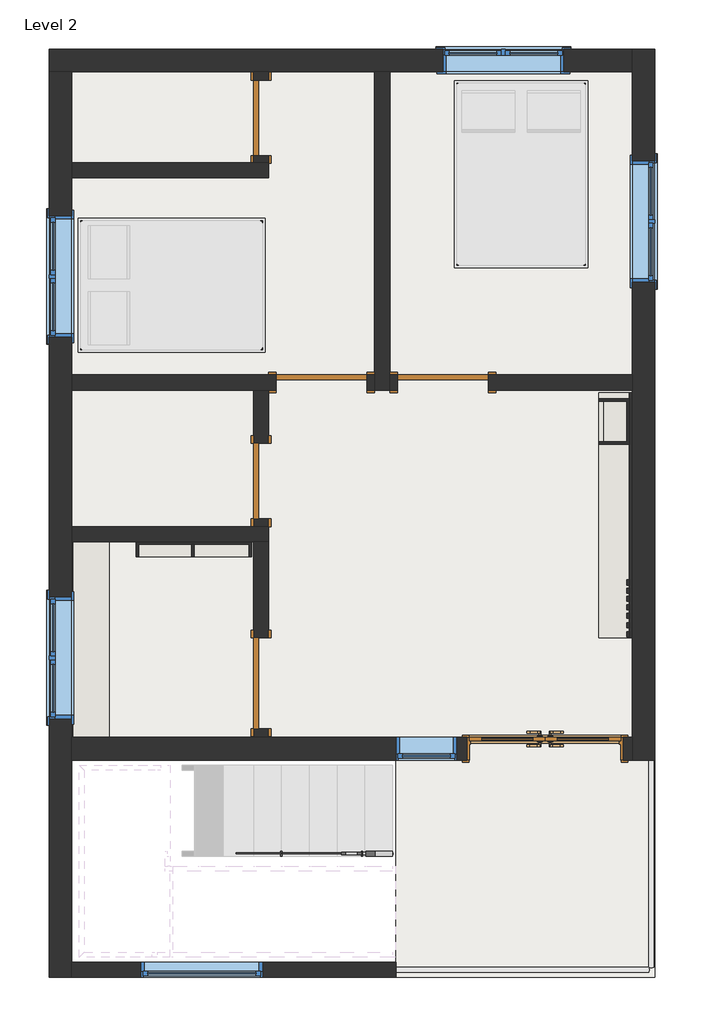
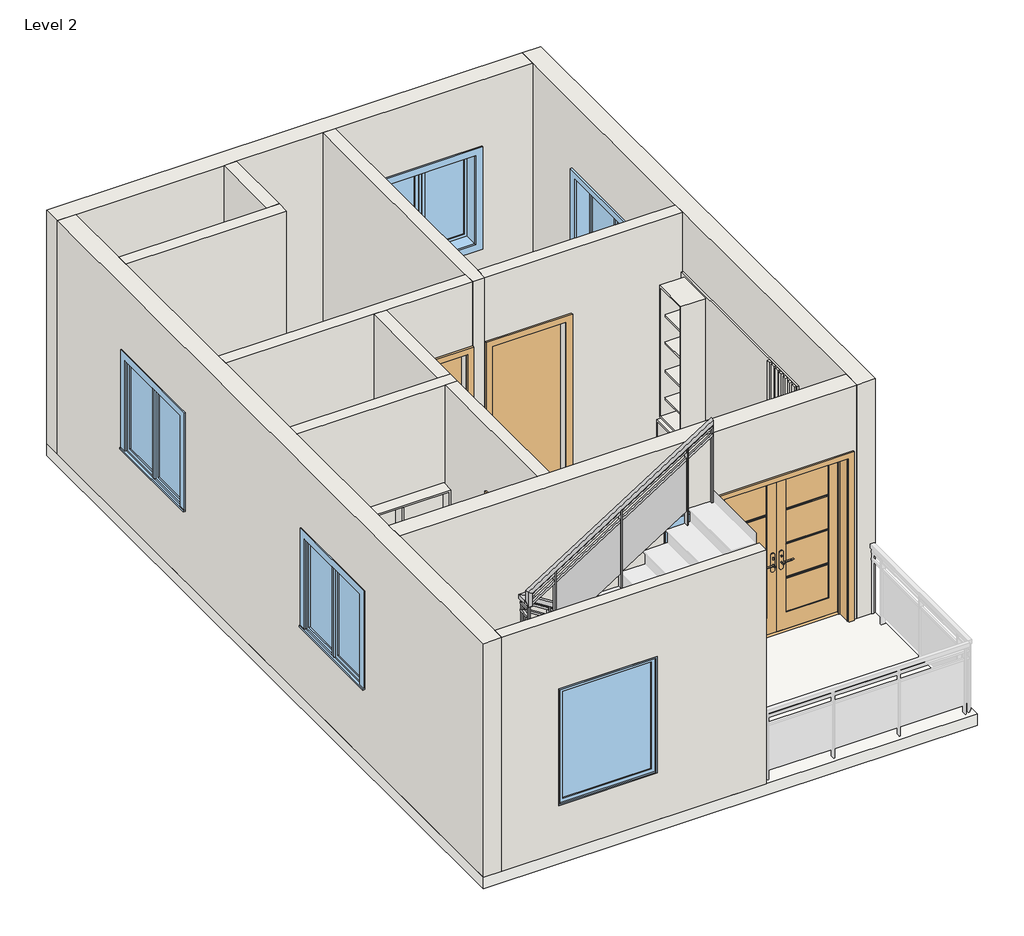
# One storey, part 1 of 2: 15 walls, 6 doors, 6 windows, 1 railing, 1 slab.
"""IFC4 building model written with IfcOpenShell, lengths in millimetres."""

from ifc_helpers import new_model, si_unit, frame, origin, place, context, project, spatial, polyline, outline, extrude, faceted_brep, transform, mapped, element, save
from components import m_door_exterior_double_full_glass_wood_clad_1524_x_2134mm_606f56d5, single_flush_2_5_e2b13fe9, door_686f89d2, door_16372e1c, walls_3_walls_1_7bd47e67, walls_4_walls_2_ccd45d7e, window_534dcd48, window_fc882ab3, fixed_4_86eadd64

model = new_model("IFC4")

# Units and contexts
model_context = context("Model", 3, world=origin())
ifc_project = project(units=[si_unit("LENGTHUNIT", "METRE", prefix="MILLI")], contexts=[model_context])

# Site, building, storey
site = spatial("IfcSite", under=ifc_project)
building = spatial("IfcBuilding", under=site)
storey = spatial("IfcBuildingStorey", under=building, Name="Level 2", Elevation=3200.4)

# Doors
placement = place(None, origin())
m_door_exterior_double_full_glass_wood_clad_1524_x_2134mm_shape = m_door_exterior_double_full_glass_wood_clad_1524_x_2134mm_606f56d5(model_context)
element("IfcDoor", 1, ObjectType="M_Door-Exterior-Double-Full Glass-Wood_Clad : 1524 x 2134mm", at=placement, inside=storey, context=model_context, shape_type="MappedRepresentation", body=[
    mapped(m_door_exterior_double_full_glass_wood_clad_1524_x_2134mm_shape, transform((-1706.0473712, -4701.782676, 3200.4), x_axis=(1.0, 0.0, 0.0), y_axis=(0.0, 1.0, 0.0), z_axis=(0.0, 0.0, 1.0))),
])
single_flush_2_5_shape = single_flush_2_5_e2b13fe9(model_context)
element("IfcDoor", 2, ObjectType="Single-Flush : 2.5'", at=placement, inside=storey, context=model_context, shape_type="MappedRepresentation", body=[
    mapped(single_flush_2_5_shape, transform((-4563.5473712, -2012.557676, 3200.4), x_axis=(0.0, -1.0, 0.0), y_axis=(1.0, 0.0, 0.0), z_axis=(0.0, 0.0, 1.0))),
])
element("IfcDoor", 3, ObjectType="Single-Flush : 2.5'", at=placement, inside=storey, context=model_context, shape_type="MappedRepresentation", body=[
    mapped(single_flush_2_5_shape, transform((-4563.5473712, 1638.692324, 3200.4), x_axis=(0.0, -1.0, 0.0), y_axis=(1.0, 0.0, 0.0), z_axis=(0.0, 0.0, 1.0))),
])
door_shape = door_686f89d2(model_context)
element("IfcDoor", 4, ObjectType="Single-Flush : 36\" x 84\"", at=placement, inside=storey, context=model_context, shape_type="MappedRepresentation", body=[
    mapped(door_shape, transform((-4563.5473712, -4044.557676, 3200.4), x_axis=(0.0, -1.0, 0.0), y_axis=(1.0, 0.0, 0.0), z_axis=(0.0, 0.0, 1.0))),
])
element("IfcDoor", 5, ObjectType="Single-Flush : 36\" x 84\"", at=placement, inside=storey, context=model_context, shape_type="MappedRepresentation", body=[
    mapped(door_shape, transform((-2734.7473712, -1021.957676, 3200.4), x_axis=(-1.0, 0.0, 0.0), y_axis=(0.0, -1.0, 0.0), z_axis=(0.0, 0.0, 1.0))),
])
door_2_shape = door_16372e1c(model_context)
element("IfcDoor", 6, ObjectType="Single-Flush : 36\" x 84\"", at=placement, inside=storey, context=model_context, shape_type="MappedRepresentation", body=[
    mapped(door_2_shape, transform((-3953.9473712, -1021.957676, 3200.4), x_axis=(1.0, 0.0, 0.0), y_axis=(0.0, 1.0, 0.0), z_axis=(0.0, 0.0, 1.0))),
])

# Railing
element("IfcRailing", 7, ObjectType="Glass Panel - Bottom Fill", at=placement, inside=storey, context=model_context, shape_type="SolidModel", body=[
    faceted_brep([(-5528.7473712, -5886.057676, 5860.4727273), (-5477.9473712, -5886.057676, 5832.586276), (-5477.9473712, -5936.857676, 5832.586276), (-5528.7473712, -5936.857676, 5860.4727273), (-3242.7473712, -5886.057676, 7315.2), (-3242.7473712, -5936.857676, 7315.2), (-3242.7473712, -5936.857676, 7254.986276), (-3242.7473712, -5886.057676, 7254.986276)], [[[0, 1, 2, 3]], [[4, 5, 6, 7]], [[1, 0, 4, 7]], [[2, 1, 7, 6]], [[3, 2, 6, 5]], [[0, 3, 5, 4]]]),
    faceted_brep([(-5477.9473712, -5886.057676, 5715.0), (-5528.7473712, -5886.057676, 5715.0), (-5528.7473712, -5936.857676, 5664.2), (-5477.9473712, -5936.857676, 5664.2), (-5477.9473712, -5860.657676, 5664.2), (-5477.9473712, -5860.657676, 5715.0), (-5528.7473712, -5860.657676, 5664.2), (-5528.7473712, -5860.657676, 5715.0), (-3242.7473712, -5784.457676, 4292.6), (-3242.7473712, -5784.457676, 4232.386276), (-3242.7473712, -5733.657676, 4232.386276), (-3242.7473712, -5733.657676, 4292.6), (-5401.7473712, -5784.457676, 5666.5090909), (-5452.5473712, -5784.457676, 5638.6226396), (-5452.5473712, -5733.657676, 5638.6226396), (-5401.7473712, -5733.657676, 5666.5090909), (-5401.7473712, -5784.457676, 5715.0), (-5452.5473712, -5784.457676, 5664.2), (-5452.5473712, -5733.657676, 5664.2), (-5401.7473712, -5733.657676, 5715.0), (-5477.9473712, -5784.457676, 5715.0), (-5477.9473712, -5784.457676, 5664.2), (-5528.7473712, -5733.657676, 5664.2), (-5528.7473712, -5733.657676, 5715.0)], [[[0, 1, 2, 3]], [[4, 5, 0, 3]], [[6, 4, 3, 2]], [[7, 6, 2, 1]], [[5, 7, 1, 0]], [[8, 9, 10, 11]], [[9, 8, 12, 13]], [[10, 9, 13, 14]], [[11, 10, 14, 15]], [[8, 11, 15, 12]], [[13, 12, 16, 17]], [[14, 13, 17, 18]], [[15, 14, 18, 19]], [[12, 15, 19, 16]], [[17, 16, 20, 21]], [[18, 17, 21, 22]], [[19, 18, 22, 23]], [[16, 19, 23, 20]], [[21, 20, 5, 4]], [[22, 21, 4, 6]], [[23, 22, 6, 7]], [[20, 23, 7, 5]]]),
    faceted_brep([(-5477.9473712, -5886.057676, 5715.0), (-5477.9473712, -5936.857676, 5664.2), (-5528.7473712, -5936.857676, 5664.2), (-5528.7473712, -5886.057676, 5715.0), (-5477.9473712, -5886.057676, 5832.586276), (-5528.7473712, -5886.057676, 5860.4727273), (-5528.7473712, -5936.857676, 5860.4727273), (-5477.9473712, -5936.857676, 5832.586276)], [[[0, 1, 2, 3]], [[4, 5, 6, 7]], [[1, 0, 4, 7]], [[2, 1, 7, 6]], [[3, 2, 6, 5]], [[0, 3, 5, 4]]]),
    faceted_brep([(-3242.7473712, -5771.757676, 4206.053431), (-3242.7473712, -5771.757676, 4175.946569), (-3242.7473712, -5746.357676, 4175.946569), (-3242.7473712, -5746.357676, 4206.053431), (-5474.2491225, -5771.757676, 5626.1), (-5481.6456199, -5771.757676, 5600.7), (-5481.6456199, -5746.357676, 5600.7), (-5474.2491225, -5746.357676, 5626.1), (-5490.6473712, -5771.757676, 5626.1), (-5490.6473712, -5771.757676, 5600.7), (-5516.0473712, -5746.357676, 5600.7), (-5516.0473712, -5746.357676, 5626.1), (-5490.6473712, -5898.757676, 5626.1), (-5516.0473712, -5898.757676, 5626.1), (-5516.0473712, -5898.757676, 5600.7), (-5490.6473712, -5898.757676, 5600.7)], [[[0, 1, 2, 3]], [[1, 0, 4, 5]], [[2, 1, 5, 6]], [[3, 2, 6, 7]], [[0, 3, 7, 4]], [[5, 4, 8, 9]], [[6, 5, 9, 10]], [[7, 6, 10, 11]], [[4, 7, 11, 8]], [[12, 13, 14, 15]], [[9, 8, 12, 15]], [[10, 9, 15, 14]], [[11, 10, 14, 13]], [[8, 11, 13, 12]]]),
    faceted_brep([(-5516.0473712, -5898.757676, 5782.0079765), (-5516.0473712, -5898.757676, 5751.9011144), (-5516.0473712, -5924.157676, 5751.9011144), (-5516.0473712, -5924.157676, 5782.0079765), (-3242.7473712, -5898.757676, 7228.653431), (-3242.7473712, -5924.157676, 7228.653431), (-3242.7473712, -5924.157676, 7198.546569), (-3242.7473712, -5898.757676, 7198.546569)], [[[0, 1, 2, 3]], [[4, 5, 6, 7]], [[1, 0, 4, 7]], [[2, 1, 7, 6]], [[3, 2, 6, 5]], [[0, 3, 5, 4]]]),
    faceted_brep([(-3242.7473712, -5771.757676, 4104.453431), (-3242.7473712, -5771.757676, 4074.346569), (-3242.7473712, -5746.357676, 4074.346569), (-3242.7473712, -5746.357676, 4104.453431), (-5474.2491225, -5771.757676, 5524.5), (-5481.6456199, -5771.757676, 5499.1), (-5481.6456199, -5746.357676, 5499.1), (-5474.2491225, -5746.357676, 5524.5), (-5490.6473712, -5771.757676, 5524.5), (-5490.6473712, -5771.757676, 5499.1), (-5516.0473712, -5746.357676, 5499.1), (-5516.0473712, -5746.357676, 5524.5), (-5490.6473712, -5898.757676, 5524.5), (-5516.0473712, -5898.757676, 5524.5), (-5516.0473712, -5898.757676, 5499.1), (-5490.6473712, -5898.757676, 5499.1)], [[[0, 1, 2, 3]], [[1, 0, 4, 5]], [[2, 1, 5, 6]], [[3, 2, 6, 7]], [[0, 3, 7, 4]], [[5, 4, 8, 9]], [[6, 5, 9, 10]], [[7, 6, 10, 11]], [[4, 7, 11, 8]], [[12, 13, 14, 15]], [[9, 8, 12, 15]], [[10, 9, 15, 14]], [[11, 10, 14, 13]], [[8, 11, 13, 12]]]),
    faceted_brep([(-5516.0473712, -5898.757676, 5680.4079765), (-5516.0473712, -5898.757676, 5650.3011144), (-5516.0473712, -5924.157676, 5650.3011144), (-5516.0473712, -5924.157676, 5680.4079765), (-3242.7473712, -5898.757676, 7127.053431), (-3242.7473712, -5924.157676, 7127.053431), (-3242.7473712, -5924.157676, 7096.946569), (-3242.7473712, -5898.757676, 7096.946569)], [[[0, 1, 2, 3]], [[4, 5, 6, 7]], [[1, 0, 4, 7]], [[2, 1, 7, 6]], [[3, 2, 6, 5]], [[0, 3, 5, 4]]]),
    extrude(outline(polyline([(7048.8999123, -3566.5973712), (6045.2, -3566.5973712), (6045.2, -3553.8973712), (7056.9817305, -3553.8973712), (7048.8999123, -3566.5973712)])), frame((0.0, -5936.857676, 0.0), z_axis=(0.0, 1.0, 0.0), x_axis=(0.0, 0.0, 1.0)), (0.0, 0.0, 1.0), 50.8),
    extrude(outline(polyline([(5710.3818182, -4373.0473712), (6227.6181818, -3560.2473712), (6894.9011144, -3560.2473712), (6377.6647508, -4373.0473712), (5710.3818182, -4373.0473712)])), frame((0.0, -5917.992833, 0.0), z_axis=(0.0, 1.0, 0.0), x_axis=(0.0, 0.0, 1.0)), (0.0, 0.0, 1.0), 6.35),
    extrude(outline(polyline([(6531.6635487, -4379.3973712), (5511.8, -4379.3973712), (5511.8, -4366.6973712), (6539.7453669, -4366.6973712), (6531.6635487, -4379.3973712)])), frame((0.0, -5936.857676, 0.0), z_axis=(0.0, 1.0, 0.0), x_axis=(0.0, 0.0, 1.0)), (0.0, 0.0, 1.0), 50.8),
    extrude(outline(polyline([(5176.9818182, -5185.8473712), (5694.2181818, -4373.0473712), (6377.6647508, -4373.0473712), (5860.4283872, -5185.8473712), (5176.9818182, -5185.8473712)])), frame((0.0, -5917.992833, 0.0), z_axis=(0.0, 1.0, 0.0), x_axis=(0.0, 0.0, 1.0)), (0.0, 0.0, 1.0), 6.35),
    extrude(outline(polyline([(6014.4271851, -5192.1973712), (5156.2, -5192.1973712), (5156.2, -5179.4973712), (6022.5090032, -5179.4973712), (6014.4271851, -5192.1973712)])), frame((0.0, -5936.857676, 0.0), z_axis=(0.0, 1.0, 0.0), x_axis=(0.0, 0.0, 1.0)), (0.0, 0.0, 1.0), 50.8),
    extrude(outline(polyline([(5464.8635487, -5179.4973712), (4445.0, -5179.4973712), (4445.0, -5166.7973712), (5456.7817305, -5166.7973712), (5464.8635487, -5179.4973712)])), frame((0.0, -5784.457676, 0.0), z_axis=(0.0, 1.0, 0.0), x_axis=(0.0, 0.0, 1.0)), (0.0, 0.0, 1.0), 50.8),
    extrude(outline(polyline([(4110.1818182, -4360.3473712), (4785.546569, -4360.3473712), (5302.7829326, -5173.1473712), (4627.4181818, -5173.1473712), (4110.1818182, -4360.3473712)])), frame((0.0, -5758.872519, 0.0), z_axis=(0.0, 1.0, 0.0), x_axis=(0.0, 0.0, 1.0)), (0.0, 0.0, 1.0), 6.35),
    extrude(outline(polyline([(4947.6271851, -4366.6973712), (4089.4, -4366.6973712), (4089.4, -4353.9973712), (4939.5453669, -4353.9973712), (4947.6271851, -4366.6973712)])), frame((0.0, -5784.457676, 0.0), z_axis=(0.0, 1.0, 0.0), x_axis=(0.0, 0.0, 1.0)), (0.0, 0.0, 1.0), 50.8),
    extrude(outline(polyline([(3576.7818182, -3547.5473712), (4268.3102054, -3547.5473712), (4785.546569, -4360.3473712), (4094.0181818, -4360.3473712), (3576.7818182, -3547.5473712)])), frame((0.0, -5758.872519, 0.0), z_axis=(0.0, 1.0, 0.0), x_axis=(0.0, 0.0, 1.0)), (0.0, 0.0, 1.0), 6.35),
    extrude(outline(polyline([(4430.3908214, -3553.8973712), (3556.0, -3553.8973712), (3556.0, -3541.1973712), (4422.3090032, -3541.1973712), (4430.3908214, -3553.8973712)])), frame((0.0, -5784.457676, 0.0), z_axis=(0.0, 1.0, 0.0), x_axis=(0.0, 0.0, 1.0)), (0.0, 0.0, 1.0), 50.8),
    extrude(outline(polyline([(-5512.8723712, -5901.932676), (-5493.8223712, -5901.932676), (-5493.8223712, -5920.982676), (-5512.8723712, -5920.982676), (-5512.8723712, -5901.932676)])), frame((0.0, 0.0, 4800.6), z_axis=(0.0, 0.0, 1.0), x_axis=(1.0, 0.0, 0.0)), (0.0, 0.0, 1.0), 863.6),
    extrude(outline(polyline([(-5493.8223712, -5768.582676), (-5512.8723712, -5768.582676), (-5512.8723712, -5749.532676), (-5493.8223712, -5749.532676), (-5493.8223712, -5768.582676)])), frame((0.0, 0.0, 4800.6), z_axis=(0.0, 0.0, 1.0), x_axis=(1.0, 0.0, 0.0)), (0.0, 0.0, 1.0), 863.6),
    extrude(outline(polyline([(-5468.4223712, -5768.582676), (-5487.4723712, -5768.582676), (-5487.4723712, -5749.532676), (-5468.4223712, -5749.532676), (-5468.4223712, -5768.582676)])), frame((0.0, 0.0, 4800.6), z_axis=(0.0, 0.0, 1.0), x_axis=(1.0, 0.0, 0.0)), (0.0, 0.0, 1.0), 863.6),
    extrude(outline(polyline([(7246.9044578, -3255.4473712), (6223.0, -3255.4473712), (6223.0, -3236.3973712), (7259.0271851, -3236.3973712), (7246.9044578, -3255.4473712)])), frame((0.0, -5920.982676, 0.0), z_axis=(0.0, 1.0, 0.0), x_axis=(0.0, 0.0, 1.0)), (0.0, 0.0, 1.0), 19.05),
    extrude(outline(polyline([(4240.4680941, -3255.4473712), (3378.2, -3255.4473712), (3378.2, -3236.3973712), (4228.3453669, -3236.3973712), (4240.4680941, -3255.4473712)])), frame((0.0, -5768.582676, 0.0), z_axis=(0.0, 1.0, 0.0), x_axis=(0.0, 0.0, 1.0)), (0.0, 0.0, 1.0), 19.05),
])

# Slab
element("IfcSlab", 8, ObjectType="6\"", at=placement, inside=storey, context=model_context, shape_type="SweptSolid", body=[
    extrude(outline(polyline([(-601.1473712, 2330.842324), (-601.1473712, -7003.657676), (-6697.1473712, -7003.657676), (-6697.1473712, 2330.842324), (-601.1473712, 2330.842324)]), holes=[polyline([(-3209.2681702, -4819.257676), (-6473.1681702, -4819.257676), (-6473.1681702, -6851.257676), (-3209.2681702, -6851.257676), (-3209.2681702, -4819.257676)])]), frame((0.0, 0.0, 3048.0), z_axis=(0.0, 0.0, 1.0), x_axis=(1.0, 0.0, 0.0)), (0.0, 0.0, 1.0), 152.4),
])

# Walls
element("IfcWall", 9, ObjectType="6\"", at=placement, inside=storey, context=model_context, shape_type="Brep", body=[
    faceted_brep([(-3420.5473712, 2102.242324, 3200.4), (-3420.5473712, -945.757676, 3200.4), (-3420.5473712, -1098.157676, 3200.4), (-3420.5473712, -1098.157676, 6248.4), (-3420.5473712, -945.757676, 6248.4), (-3420.5473712, 2102.242324, 6248.4), (-3268.1473712, 2102.242324, 3200.4), (-3268.1473712, 2102.242324, 6248.4), (-3268.1473712, -945.757676, 6248.4), (-3268.1473712, -1098.157676, 6248.4), (-3268.1473712, -1098.157676, 3200.4), (-3268.1473712, -945.757676, 3200.4)], [[[0, 1, 2, 3, 4, 5]], [[6, 7, 8, 9, 10, 11]], [[2, 1, 0, 6, 11, 10]], [[5, 4, 3, 9, 8, 7]], [[0, 5, 7, 6]], [[3, 2, 10, 9]]]),
])
element("IfcWall", 10, ObjectType="6\"", at=placement, inside=storey, context=model_context, shape_type="Brep", body=[
    faceted_brep([(-3420.5473712, -945.757676, 3200.4), (-3496.7473712, -945.757676, 3200.4), (-3496.7473712, -945.757676, 5334.0), (-4411.1473712, -945.757676, 5334.0), (-4411.1473712, -945.757676, 3200.4), (-6468.5473712, -945.757676, 3200.4), (-6468.5473712, -945.757676, 6248.4), (-3420.5473712, -945.757676, 6248.4), (-3496.7473712, -1098.157676, 5334.0), (-3496.7473712, -1098.157676, 3200.4), (-3420.5473712, -1098.157676, 3200.4), (-3420.5473712, -1098.157676, 6248.4), (-4487.3473712, -1098.157676, 6248.4), (-4639.7473712, -1098.157676, 6248.4), (-6468.5473712, -1098.157676, 6248.4), (-6468.5473712, -1098.157676, 3200.4), (-4639.7473712, -1098.157676, 3200.4), (-4487.3473712, -1098.157676, 3200.4), (-4411.1473712, -1098.157676, 3200.4), (-4411.1473712, -1098.157676, 5334.0)], [[[0, 1, 2, 3, 4, 5, 6, 7]], [[8, 9, 10, 11, 12, 13, 14, 15, 16, 17, 18, 19]], [[10, 9, 1, 0]], [[18, 17, 16, 15, 5, 4]], [[7, 6, 14, 13, 12, 11]], [[6, 5, 15, 14]], [[0, 7, 11, 10]], [[2, 1, 9, 8]], [[3, 2, 8, 19]], [[4, 3, 19, 18]]]),
])
element("IfcWall", 11, ObjectType="6\"", at=placement, inside=storey, context=model_context, shape_type="SweptSolid", body=[
    extrude(outline(polyline([(3200.4, -3268.1473712), (3200.4, -3191.9473712), (5334.0, -3191.9473712), (5334.0, -2277.5473712), (3200.4, -2277.5473712), (3200.4, -829.7473712), (6248.4, -829.7473712), (6248.4, -3268.1473712), (3200.4, -3268.1473712)])), frame((0.0, -1098.157676, 0.0), z_axis=(0.0, 1.0, 0.0), x_axis=(0.0, 0.0, 1.0)), (0.0, 0.0, 1.0), 152.4),
])
element("IfcWall", 12, ObjectType="6\"", at=placement, inside=storey, context=model_context, shape_type="Brep", body=[
    faceted_brep([(-6468.5473712, -2622.157676, 3200.4), (-4639.7473712, -2622.157676, 3200.4), (-4487.3473712, -2622.157676, 3200.4), (-4487.3473712, -2622.157676, 6248.4), (-4639.7473712, -2622.157676, 6248.4), (-6468.5473712, -2622.157676, 6248.4), (-6468.5473712, -2469.757676, 3200.4), (-6468.5473712, -2469.757676, 6248.4), (-4639.7473712, -2469.757676, 6248.4), (-4487.3473712, -2469.757676, 6248.4), (-4487.3473712, -2469.757676, 3200.4), (-4639.7473712, -2469.757676, 3200.4)], [[[0, 1, 2, 3, 4, 5]], [[6, 7, 8, 9, 10, 11]], [[2, 1, 0, 6, 11, 10]], [[5, 4, 3, 9, 8, 7]], [[0, 5, 7, 6]], [[3, 2, 10, 9]]]),
])
element("IfcWall", 13, ObjectType="6\"", at=placement, inside=storey, context=model_context, shape_type="SweptSolid", body=[
    extrude(outline(polyline([(-2393.557676, 5334.0), (-2393.557676, 3200.4), (-2469.757676, 3200.4), (-2469.757676, 6248.4), (-1098.157676, 6248.4), (-1098.157676, 3200.4), (-1631.557676, 3200.4), (-1631.557676, 5334.0), (-2393.557676, 5334.0)])), frame((-4639.7473712, 0.0, 0.0), z_axis=(1.0, 0.0, 0.0), x_axis=(0.0, 1.0, 0.0)), (0.0, 0.0, 1.0), 152.4),
])
element("IfcWall", 14, ObjectType="6\"", at=placement, inside=storey, context=model_context, shape_type="SweptSolid", body=[
    extrude(outline(polyline([(-4501.757676, 5334.0), (-4501.757676, 3200.4), (-4590.657676, 3200.4), (-4590.657676, 6248.4), (-2622.157676, 6248.4), (-2622.157676, 3200.4), (-3587.357676, 3200.4), (-3587.357676, 5334.0), (-4501.757676, 5334.0)])), frame((-4639.7473712, 0.0, 0.0), z_axis=(1.0, 0.0, 0.0), x_axis=(0.0, 1.0, 0.0)), (0.0, 0.0, 1.0), 152.4),
])
element("IfcWall", 15, ObjectType="6\"", at=placement, inside=storey, context=model_context, shape_type="SweptSolid", body=[
    extrude(outline(polyline([(1257.692324, 5334.0), (1257.692324, 3200.4), (1187.842324, 3200.4), (1187.842324, 6248.4), (2102.242324, 6248.4), (2102.242324, 3200.4), (2019.692324, 3200.4), (2019.692324, 5334.0), (1257.692324, 5334.0)])), frame((-4639.7473712, 0.0, 0.0), z_axis=(1.0, 0.0, 0.0), x_axis=(0.0, 1.0, 0.0)), (0.0, 0.0, 1.0), 152.4),
])
element("IfcWall", 16, ObjectType="6\"", at=placement, inside=storey, context=model_context, shape_type="Brep", body=[
    faceted_brep([(-4487.3473712, 1187.842324, 3200.4), (-4639.7473712, 1187.842324, 3200.4), (-6468.5473712, 1187.842324, 3200.4), (-6468.5473712, 1187.842324, 6248.4), (-4639.7473712, 1187.842324, 6248.4), (-4487.3473712, 1187.842324, 6248.4), (-4487.3473712, 1035.442324, 3200.4), (-4487.3473712, 1035.442324, 6248.4), (-6468.5473712, 1035.442324, 6248.4), (-6468.5473712, 1035.442324, 3200.4)], [[[0, 1, 2, 3, 4, 5]], [[6, 7, 8, 9]], [[2, 1, 0, 6, 9]], [[5, 4, 3, 8, 7]], [[3, 2, 9, 8]], [[0, 5, 7, 6]]]),
])
element("IfcWall", 17, ObjectType="6\"", at=placement, inside=storey, context=model_context, shape_type="SweptSolid", body=[
    extrude(outline(polyline([(3200.4, -3204.6473712), (6248.4, -3204.6473712), (6248.4, -6468.5473712), (3200.4, -6468.5473712), (3200.4, -3204.6473712)]), holes=[polyline([(5334.0, -5770.0473712), (5334.0, -4550.8473712), (3810.0, -4550.8473712), (3810.0, -5770.0473712), (5334.0, -5770.0473712)])]), frame((0.0, -7003.657676, 0.0), z_axis=(0.0, 1.0, 0.0), x_axis=(0.0, 0.0, 1.0)), (0.0, 0.0, 1.0), 152.4),
])
element("IfcWall", 18, ObjectType="9\"", at=placement, inside=storey, context=model_context, shape_type="Brep", body=[
    faceted_brep([(-6697.1473712, 2102.242324, 3200.4), (-6468.5473712, 2102.242324, 3200.4), (-4639.7473712, 2102.242324, 3200.4), (-4487.3473712, 2102.242324, 3200.4), (-3420.5473712, 2102.242324, 3200.4), (-3268.1473712, 2102.242324, 3200.4), (-829.7473712, 2102.242324, 3200.4), (-829.7473712, 2102.242324, 6248.4), (-3268.1473712, 2102.242324, 6248.4), (-3420.5473712, 2102.242324, 6248.4), (-4487.3473712, 2102.242324, 6248.4), (-4639.7473712, 2102.242324, 6248.4), (-6468.5473712, 2102.242324, 6248.4), (-6697.1473712, 2102.242324, 6248.4), (-1515.5473712, 2102.242324, 5334.0), (-1515.5473712, 2102.242324, 4114.8), (-2734.7473712, 2102.242324, 4114.8), (-2734.7473712, 2102.242324, 5334.0), (-6697.1473712, 2330.842324, 3200.4), (-6697.1473712, 2330.842324, 6248.4), (-829.7473712, 2330.842324, 6248.4), (-829.7473712, 2330.842324, 3200.4), (-1515.5473712, 2330.842324, 5334.0), (-2734.7473712, 2330.842324, 5334.0), (-2734.7473712, 2330.842324, 4114.8), (-1515.5473712, 2330.842324, 4114.8)], [[[0, 1, 2, 3, 4, 5, 6, 7, 8, 9, 10, 11, 12, 13], [14, 15, 16, 17]], [[18, 19, 20, 21], [22, 23, 24, 25]], [[6, 5, 4, 3, 2, 1, 0, 18, 21]], [[13, 12, 11, 10, 9, 8, 7, 20, 19]], [[0, 13, 19, 18]], [[7, 6, 21, 20]], [[15, 14, 22, 25]], [[16, 15, 25, 24]], [[17, 16, 24, 23]], [[14, 17, 23, 22]]]),
])
element("IfcWall", 19, ObjectType="9\"", at=placement, inside=storey, context=model_context, shape_type="Brep", body=[
    faceted_brep([(-6468.5473712, -7003.657676, 3200.4), (-6468.5473712, -6851.257676, 3200.4), (-6468.5473712, -4819.257676, 3200.4), (-6468.5473712, -4590.657676, 3200.4), (-6468.5473712, -2622.157676, 3200.4), (-6468.5473712, -2469.757676, 3200.4), (-6468.5473712, -1098.157676, 3200.4), (-6468.5473712, -945.757676, 3200.4), (-6468.5473712, 1035.442324, 3200.4), (-6468.5473712, 1187.842324, 3200.4), (-6468.5473712, 2102.242324, 3200.4), (-6468.5473712, 2102.242324, 6248.4), (-6468.5473712, 1187.842324, 6248.4), (-6468.5473712, 1035.442324, 6248.4), (-6468.5473712, -945.757676, 6248.4), (-6468.5473712, -1098.157676, 6248.4), (-6468.5473712, -2469.757676, 6248.4), (-6468.5473712, -2622.157676, 6248.4), (-6468.5473712, -4590.657676, 6248.4), (-6468.5473712, -4819.257676, 6248.4), (-6468.5473712, -6851.257676, 6248.4), (-6468.5473712, -7003.657676, 6248.4), (-6468.5473712, -3180.957676, 5334.0), (-6468.5473712, -3180.957676, 4114.8), (-6468.5473712, -4400.157676, 4114.8), (-6468.5473712, -4400.157676, 5334.0), (-6468.5473712, 654.442324, 5334.0), (-6468.5473712, 654.442324, 4114.8), (-6468.5473712, -564.757676, 4114.8), (-6468.5473712, -564.757676, 5334.0), (-6697.1473712, -7003.657676, 3200.4), (-6697.1473712, -7003.657676, 6248.4), (-6697.1473712, 2102.242324, 6248.4), (-6697.1473712, 2102.242324, 3200.4), (-6697.1473712, -3180.957676, 5334.0), (-6697.1473712, -4400.157676, 5334.0), (-6697.1473712, -4400.157676, 4114.8), (-6697.1473712, -3180.957676, 4114.8), (-6697.1473712, 654.442324, 5334.0), (-6697.1473712, -564.757676, 5334.0), (-6697.1473712, -564.757676, 4114.8), (-6697.1473712, 654.442324, 4114.8)], [[[0, 1, 2, 3, 4, 5, 6, 7, 8, 9, 10, 11, 12, 13, 14, 15, 16, 17, 18, 19, 20, 21], [22, 23, 24, 25], [26, 27, 28, 29]], [[30, 31, 32, 33], [34, 35, 36, 37], [38, 39, 40, 41]], [[10, 9, 8, 7, 6, 5, 4, 3, 2, 1, 0, 30, 33]], [[21, 20, 19, 18, 17, 16, 15, 14, 13, 12, 11, 32, 31]], [[0, 21, 31, 30]], [[11, 10, 33, 32]], [[23, 22, 34, 37]], [[24, 23, 37, 36]], [[25, 24, 36, 35]], [[22, 25, 35, 34]], [[27, 26, 38, 41]], [[28, 27, 41, 40]], [[29, 28, 40, 39]], [[26, 29, 39, 38]]]),
])
element("IfcWall", 20, ObjectType="9\"", at=placement, inside=storey, context=model_context, shape_type="Brep", body=[
    faceted_brep([(-829.7473712, 2330.842324, 3200.4), (-829.7473712, 2102.242324, 3200.4), (-829.7473712, -945.757676, 3200.4), (-829.7473712, -1098.157676, 3200.4), (-829.7473712, -4590.657676, 3200.4), (-829.7473712, -4819.257676, 3200.4), (-829.7473712, -4819.257676, 6248.4), (-829.7473712, -4590.657676, 6248.4), (-829.7473712, -1098.157676, 6248.4), (-829.7473712, -945.757676, 6248.4), (-829.7473712, 2102.242324, 6248.4), (-829.7473712, 2330.842324, 6248.4), (-829.7473712, -12.307676, 5334.0), (-829.7473712, -12.307676, 4114.8), (-829.7473712, 1206.892324, 4114.8), (-829.7473712, 1206.892324, 5334.0), (-601.1473712, 2330.842324, 3200.4), (-601.1473712, 2330.842324, 6248.4), (-601.1473712, -4819.257676, 6248.4), (-601.1473712, -4819.257676, 3200.4), (-601.1473712, -12.307676, 5334.0), (-601.1473712, 1206.892324, 5334.0), (-601.1473712, 1206.892324, 4114.8), (-601.1473712, -12.307676, 4114.8)], [[[0, 1, 2, 3, 4, 5, 6, 7, 8, 9, 10, 11], [12, 13, 14, 15]], [[16, 17, 18, 19], [20, 21, 22, 23]], [[5, 4, 3, 2, 1, 0, 16, 19]], [[6, 5, 19, 18]], [[11, 10, 9, 8, 7, 6, 18, 17]], [[0, 11, 17, 16]], [[13, 12, 20, 23]], [[14, 13, 23, 22]], [[15, 14, 22, 21]], [[12, 15, 21, 20]]]),
])
element("IfcWall", 21, ObjectType="9\"", at=placement, inside=storey, context=model_context, shape_type="Brep", body=[
    faceted_brep([(-829.7473712, -4819.257676, 6248.4), (-6468.5473712, -4819.257676, 6248.4), (-6468.5473712, -4819.257676, 3200.4), (-2493.0473712, -4819.257676, 3200.4), (-2493.0473712, -4819.257676, 5359.0), (-919.0473712, -4819.257676, 5359.0), (-919.0473712, -4819.257676, 3200.4), (-829.7473712, -4819.257676, 3200.4), (-3204.6473712, -4819.257676, 5334.0), (-2595.0473712, -4819.257676, 5334.0), (-2595.0473712, -4819.257676, 3505.2), (-3204.6473712, -4819.257676, 3505.2), (-6468.5473712, -4590.657676, 6248.4), (-4639.7473712, -4590.657676, 6248.4), (-4487.3473712, -4590.657676, 6248.4), (-829.7473712, -4590.657676, 6248.4), (-829.7473712, -4590.657676, 3200.4), (-919.0473712, -4590.657676, 3200.4), (-919.0473712, -4590.657676, 5359.0), (-2493.0473712, -4590.657676, 5359.0), (-2493.0473712, -4590.657676, 3200.4), (-4487.3473712, -4590.657676, 3200.4), (-4639.7473712, -4590.657676, 3200.4), (-6468.5473712, -4590.657676, 3200.4), (-3204.6473712, -4590.657676, 5334.0), (-3204.6473712, -4590.657676, 3505.2), (-2595.0473712, -4590.657676, 3505.2), (-2595.0473712, -4590.657676, 5334.0)], [[[0, 1, 2, 3, 4, 5, 6, 7], [8, 9, 10, 11]], [[12, 13, 14, 15, 16, 17, 18, 19, 20, 21, 22, 23], [24, 25, 26, 27]], [[2, 23, 22, 21, 20, 3]], [[16, 7, 6, 17]], [[1, 0, 15, 14, 13, 12]], [[2, 1, 12, 23]], [[0, 7, 16, 15]], [[5, 18, 17, 6]], [[18, 5, 4, 19]], [[19, 4, 3, 20]], [[25, 24, 8, 11]], [[26, 25, 11, 10]], [[27, 26, 10, 9]], [[24, 27, 9, 8]]]),
])
walls_3_walls_1_shape = walls_3_walls_1_7bd47e67(model_context)
element("IfcWall", 22, ObjectType="Walls 3 : Walls 1", at=placement, inside=storey, context=model_context, shape_type="MappedRepresentation", body=[
    mapped(walls_3_walls_1_shape, transform((0.0, 0.0, 0.0), x_axis=(1.0, 0.0, 0.0), y_axis=(0.0, 1.0, 0.0), z_axis=(0.0, 0.0, 1.0))),
])
walls_4_walls_2_shape = walls_4_walls_2_ccd45d7e(model_context)
element("IfcWall", 23, ObjectType="Walls 4 : Walls 2", at=placement, inside=storey, context=model_context, shape_type="MappedRepresentation", body=[
    mapped(walls_4_walls_2_shape, transform((0.0, 0.0, 0.0), x_axis=(1.0, 0.0, 0.0), y_axis=(0.0, 1.0, 0.0), z_axis=(0.0, 0.0, 1.0))),
])

# Windows
window_shape = window_534dcd48(model_context)
element("IfcWindow", 24, ObjectType="Casement Dbl with Trim : 48\" x 48\"", at=placement, inside=storey, context=model_context, shape_type="MappedRepresentation", body=[
    mapped(window_shape, transform((-6563.7973712, -3790.557676, 3200.4), x_axis=(0.0, 1.0, 0.0), y_axis=(-1.0, 0.0, 0.0), z_axis=(0.0, 0.0, 1.0))),
])
element("IfcWindow", 25, ObjectType="Casement Dbl with Trim : 48\" x 48\"", at=placement, inside=storey, context=model_context, shape_type="MappedRepresentation", body=[
    mapped(window_shape, transform((-734.4973712, 597.292324, 3200.4), x_axis=(0.0, -1.0, 0.0), y_axis=(1.0, 0.0, 0.0), z_axis=(0.0, 0.0, 1.0))),
])
element("IfcWindow", 26, ObjectType="Casement Dbl with Trim : 48\" x 48\"", at=placement, inside=storey, context=model_context, shape_type="MappedRepresentation", body=[
    mapped(window_shape, transform((-2125.1473712, 2197.492324, 3200.4), x_axis=(1.0, 0.0, 0.0), y_axis=(0.0, 1.0, 0.0), z_axis=(0.0, 0.0, 1.0))),
])
element("IfcWindow", 27, ObjectType="Casement Dbl with Trim : 48\" x 48\"", at=placement, inside=storey, context=model_context, shape_type="MappedRepresentation", body=[
    mapped(window_shape, transform((-6563.7973712, 44.842324, 3200.4), x_axis=(0.0, 1.0, 0.0), y_axis=(-1.0, 0.0, 0.0), z_axis=(0.0, 0.0, 1.0))),
])
window_2_shape = window_fc882ab3(model_context)
element("IfcWindow", 28, ObjectType="Fixed : 24\" x 72\"", at=placement, inside=storey, context=model_context, shape_type="MappedRepresentation", body=[
    mapped(window_2_shape, transform((-2937.9473712, -4704.957676, 3200.4), x_axis=(-1.0, 0.0, 0.0), y_axis=(0.0, -1.0, 0.0), z_axis=(0.0, 0.0, 1.0))),
])
fixed_4_shape = fixed_4_86eadd64(model_context)
element("IfcWindow", 29, ObjectType="Fixed : 4'", at=placement, inside=storey, context=model_context, shape_type="MappedRepresentation", body=[
    mapped(fixed_4_shape, transform((-5198.5473712, -6927.457676, 3200.4), x_axis=(-1.0, 0.0, 0.0), y_axis=(0.0, -1.0, 0.0), z_axis=(0.0, 0.0, 1.0))),
])

save(model, "model.ifc")

# Revit data of these elements
# Type "M_Door-Exterior-Double-Full Glass-Wood_Clad : 1524 x 2134mm"
#   Type Mark = "9"
#   Assembly Code = "B2030100"
#   Analytic Construction = "French door, wood frame with double glass"
#   Top Rail = 0' - 4.72441"
#   Threshold Offset [instance default] = 0' - 0.59055"
#   Thickness = 0' - 1.37795"
#   Thermal Resistance (R) = 1.9158 (h·ft²·°F)/BTU
#   Swing Angle [instance default] = 90.00°
#   Stiles = 0' - 4.72441"
#   Rough Width = 5' - 1.9685"
#   Rough Height = 7' - 0.98425"
#   Panel Width = 2' - 6"
#   Door Offset [instance default] = 0' - 0"
#   Height = 7' - 0"
#   Width = 5' - 0"
#   Heat Transfer Coefficient (U) = 0.5220 BTU/(h·ft²·°F)
#   Bottom Rail = 0' - 9.05512"
#   Exterior Trim [instance default] = yes
#   Threshold [instance default] = yes
#   Show Grill [instance default] = yes
#   Function = 1
#   Trim Material = Cherry
#   Threshold Material = Cherry
#   Panel Material = Cherry
#   Glazing = Glass
#   Frame Material = Cherry
#   Door Handle Material = Aluminum
#   Visual Light Transmittance = 0
#   Solar Heat Gain Coefficient = 0
#   Wall Closure = (empty or 0)
#   Construction Type = (empty or 0)
# Type "Single-Flush : 2.5'"
#   Type Mark = "8"
#   Construction Type Id = "MDOOR"
#   Assembly Code = "C1020"
#   Analytic Construction = "Metal"
#   Thickness = 0' - 2"
#   Heat Transfer Coefficient (U) = 0.651978 BTU/(h·ft²·°F)
#   Height = 7' - 0"
#   Trim Projection Ext = 0' - 1"
#   Trim Projection Int = 0' - 1"
#   Trim Width = 0' - 3"
#   Width = 2' - 6"
#   Define Thermal Properties by = 1
#   Door Material = Door - Panel
#   Frame Material = Door - Frame
#   Visual Light Transmittance = 0
#   Solar Heat Gain Coefficient = 0
#   Function = (empty or 0)
#   Wall Closure = (empty or 0)
# Type "Single-Flush : 36\" x 84\""
#   Type Mark = "1"
#   Construction Type Id = "MDOOR"
#   Assembly Code = "C1020"
#   Analytic Construction = "Metal"
#   Thickness = 0' - 2"
#   Heat Transfer Coefficient (U) = 0.651978 BTU/(h·ft²·°F)
#   Height = 7' - 0"
#   Trim Projection Ext = 0' - 1"
#   Trim Projection Int = 0' - 1"
#   Trim Width = 0' - 3"
#   Width = 3' - 0"
#   Define Thermal Properties by = 1
#   Door Material = Door - Panel
#   Frame Material = Door - Frame
#   Visual Light Transmittance = 0
#   Solar Heat Gain Coefficient = 0
#   Function = (empty or 0)
#   Wall Closure = (empty or 0)
# Type "Glass Panel - Bottom Fill"
#   Assembly Code = "C2010400"
#   built-in parameter 1008612 = 0.0416667 (stored number, unit not read)
#   built-in parameter 1008611 = 0.0416667 (stored number, unit not read)
#   built-in parameter 1008609 = 0.333333 (stored number, unit not read)
#   built-in parameter 1008604 = 0.166667 (stored number, unit not read)
#   built-in parameter 1008603 = 0.166667 (stored number, unit not read)
#   Railing Height = 3' - 0"
#   built-in parameter 1008630 = 2
#   built-in parameter 1008610 = 2
#   built-in parameter 1008618 = Baluster - Square : 3/4"
# Type "6\""
#   Assembly Code = "B1010"
#   Function = 0
#   Layers, outside or top first: 0' - 6" "floor" (function 1)
# Type "6\""
#   Assembly Code = "B2010"
#   Layers, outside or top first: 0' - 6" "ext wall" (function 1)
# Type "9\""
#   Assembly Code = "B2010"
#   Layers, outside or top first: 0' - 9" "int wall" (function 1)
# Type "Casement Dbl with Trim : 48\" x 48\""
#   Type Mark = "10"
#   Construction Type Id = "GSP4R"
#   Assembly Code = "B2020100"
#   Analytic Construction = "1/8 in Pilkington single glazing"
#   Visual Light Transmittance = 0.9
#   Solar Heat Gain Coefficient = 0.78
#   Heat Transfer Coefficient (U) = 0.6496 BTU/(h·ft²·°F)
#   Height = 4' - 0"
#   Default Sill Height = 3' - 0"
#   Trim Projection - Ext. = 0' - 0 1/2"
#   Trim Projection - Int. = 0' - 0 3/4"
#   Trim Width - Exterior = 0' - 3 1/2"
#   Trim Width - Interior = 0' - 3 1/2"
#   Width = 4' - 0"
#   Window Inset = 0' - 0 3/4"
#   Define Thermal Properties by = 1
#   Glass Pane Material = Glass
#   Sash Material = Sash
#   Trim Exterior Material = Trim
#   Trim Interior Material = Trim
#   Wall Closure = (empty or 0)
# Type "Fixed : 24\" x 72\""
#   Type Mark = "7"
#   Construction Type Id = "GSP4R"
#   Assembly Code = "B2020100"
#   Analytic Construction = "1/8 in Pilkington single glazing"
#   Visual Light Transmittance = 0.9
#   Solar Heat Gain Coefficient = 0.78
#   Heat Transfer Coefficient (U) = 0.6496 BTU/(h·ft²·°F)
#   Height = 6' - 0"
#   Default Sill Height = 1' - 0"
#   Width = 2' - 0"
#   Window Inset = 0' - 0 3/4"
#   Define Thermal Properties by = 1
#   Glass Pane Material = Glass
#   Sash Material = Sash
#   Wall Closure = (empty or 0)
# Type "Fixed : 4'"
#   Type Mark = "13"
#   Construction Type Id = "GSP4R"
#   Assembly Code = "B2020100"
#   Analytic Construction = "1/8 in Pilkington single glazing"
#   Visual Light Transmittance = 0.9
#   Solar Heat Gain Coefficient = 0.78
#   Heat Transfer Coefficient (U) = 0.6496 BTU/(h·ft²·°F)
#   Height = 5' - 0"
#   Default Sill Height = 2' - 0"
#   Width = 4' - 0"
#   Window Inset = 0' - 0 3/4"
#   Define Thermal Properties by = 1
#   Glass Pane Material = Glass
#   Sash Material = Sash
#   Wall Closure = (empty or 0)
# Element 1 (IfcDoor, "M_Door-Exterior-Double-Full Glass-Wood_Clad : 1524 x 2134mm")
#   Threshold Offset = 0' - 0.59055"
#   Swing Angle = 90.00°
#   Door Offset = 0' - 0"
#   Threshold = yes
#   Show Grill = yes
#   Exterior Trim = yes
#   Phase Created = New Construction
#   Materials on its faces: "Cherry", "Aluminum", "Glass"
# Elements 2, 3 (IfcDoor, "Single-Flush : 2.5'")
#   Phase Created = New Construction
#   Materials on its faces: "Door - Frame", "Door - Panel"
# Elements 4, 5, 6 (IfcDoor, "Single-Flush : 36\" x 84\"")
#   Phase Created = New Construction
#   Materials on its faces: "Door - Frame", "Door - Panel"
# Element 7 (IfcRailing, "Glass Panel - Bottom Fill")
#   Phase Created = New Construction
#   Materials on its faces: "Glass"
# Element 8 (IfcSlab, "6\"")
#   Height Offset From Level = 0' - 0"
#   Phase Created = New Construction
#   Materials on its faces: "floor"
# Elements 9, 10, 11, 12, 13, 14, 15, 16, 17 (IfcWall, "6\"")
#   Top Offset = 0' - 0"
#   Base Offset = 0' - 0"
#   Unconnected Height = 10' - 0"
#   wall height = 10' - 0"
#   Phase Created = New Construction
#   Base Constraint = Level 2
#   Materials on its faces: "ext wall"
# Elements 18, 20, 21 (IfcWall, "9\"")
#   Top Offset = 0' - 0"
#   Base Offset = 0' - 0"
#   Unconnected Height = 10' - 0"
#   wall height = 10' - 0"
#   Phase Created = New Construction
#   Base Constraint = Level 2
#   Materials on its faces: "int wall"
# Element 19 (IfcWall, "9\"")
#   Top Offset = 0' - 0"
#   Base Offset = 0' - 0"
#   Unconnected Height = 10' - 0"
#   wall height = 10' - 0"
#   Phase Created = New Construction
#   Base Constraint = Level 2
#   Materials on its faces: "int wall", "ext wall"
# Element 22 (IfcWall, "Walls 3 : Walls 1")
#   Phase Created = New Construction
#   Materials on its faces: "drawers", "wood", "clear glass", "stone", "Default Wall"
# Element 23 (IfcWall, "Walls 4 : Walls 2")
#   Phase Created = New Construction
#   Materials on its faces: "drawers", "metal", "wood"
# Element 24 (IfcWindow, "Casement Dbl with Trim : 48\" x 48\"")
#   Mark = "7"
#   Phase Created = New Construction
#   Materials on its faces: "Sash", "Trim", "Glass"
# Element 25 (IfcWindow, "Casement Dbl with Trim : 48\" x 48\"")
#   Mark = "8"
#   Phase Created = New Construction
#   Materials on its faces: "Sash", "Trim", "Glass"
# Element 26 (IfcWindow, "Casement Dbl with Trim : 48\" x 48\"")
#   Mark = "9"
#   Phase Created = New Construction
#   Materials on its faces: "Sash", "Trim", "Glass"
# Element 27 (IfcWindow, "Casement Dbl with Trim : 48\" x 48\"")
#   Mark = "22"
#   Phase Created = New Construction
#   Materials on its faces: "Sash", "Trim", "Glass"
# Element 28 (IfcWindow, "Fixed : 24\" x 72\"")
#   Mark = "10"
#   Phase Created = New Construction
#   Materials on its faces: "Sash", "Glass"
# Element 29 (IfcWindow, "Fixed : 4'")
#   Mark = "18"
#   Phase Created = New Construction
#   Materials on its faces: "Sash", "Glass"
# Materials
#   "Cherry": class "Wood", colour RGB 226 177 128, transparency 0, Description = "Prunus Serotina", Cost = 0
#   "Glass": class "Glass", colour RGB 0 128 192, transparency 0.75, Description = "Soda Lime Glass", Cost = 0
#   "Aluminum": class "Metal", colour RGB 247 247 247, transparency 0, Description = "Aluminum 6061", Cost = 0
#   "Door - Panel": class "Wood", colour RGB 210 159 95, transparency 0
#   "Door - Frame": colour RGB 118 70 51, transparency 0
#   "floor": class "Generic", colour RGB 138 129 123, transparency 0, Cost = 0
#   "ext wall": class "Generic", colour RGB 219 210 180, transparency 0, Cost = 0
#   "int wall": class "Generic", colour RGB 230 213 172, transparency 0, Cost = 0
#   "Sash": class "Wood", colour RGB 224 178 126, transparency 0
#   "Trim": class "Wood", colour RGB 224 178 126, transparency 0
#   "drawers": class "Generic", colour RGB 121 66 39, transparency 0, Cost = 0
#   "wood": class "Generic", colour RGB 255 226 181, transparency 0, Cost = 0
#   "clear glass": class "Generic", colour RGB 141 181 235, transparency 0.9, Cost = 0
#   "stone": class "Generic", colour RGB 125 126 130, transparency 0, Cost = 0
#   "Default Wall": colour RGB 128 128 128, transparency 0
#   "metal": class "Generic", colour RGB 76 25 7, transparency 0, Cost = 0
